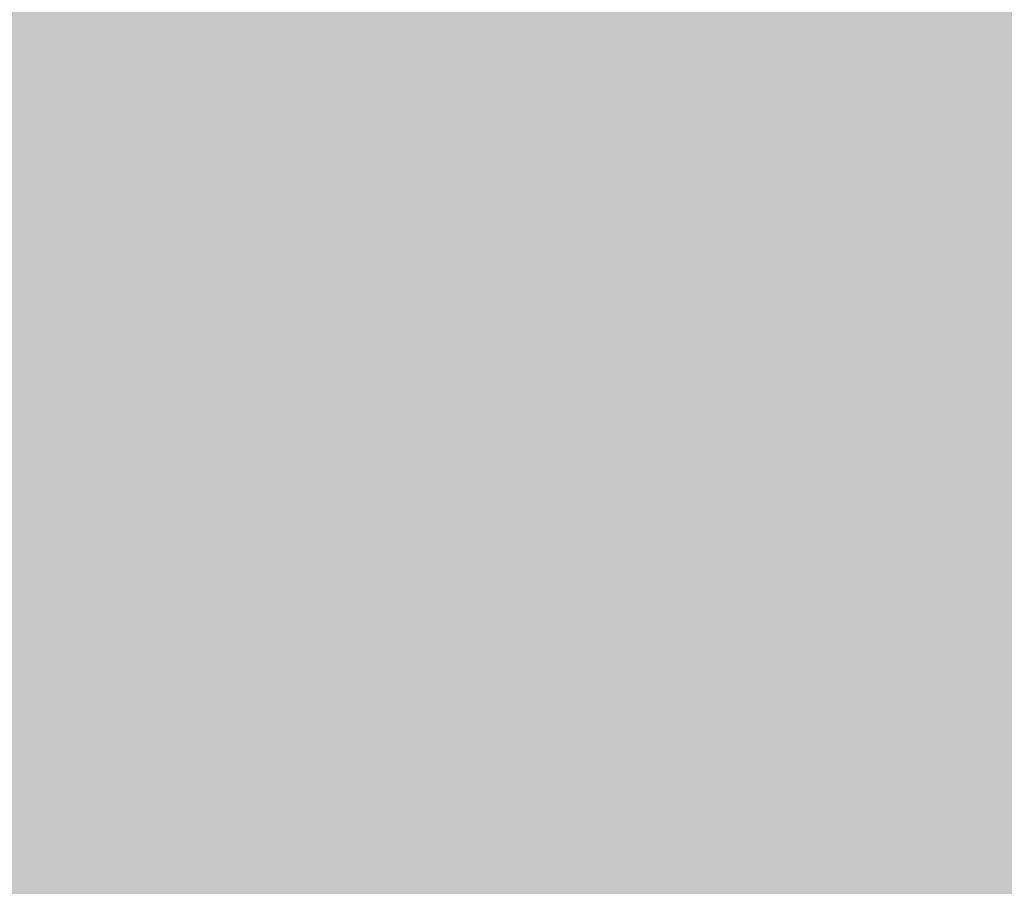
# Model space of a CAD drawing. Units: feet. Extents: x 3168 to 4724, y 827 to 1477.
# Tile 99 of 256: x 3277.376 to 3284.479, y 1087.401 to 1093.654. Entities that reach past the tile are written whole.
import ezdxf

# ---------------------------------------------------------------- set-up
doc = ezdxf.new("R2010")
doc.units = ezdxf.units.FT
doc.layers.add('A-ELEV-PATT', color=8, linetype='Continuous', lineweight=13)

msp = doc.modelspace()

# ---------------------------------------------------------------- hatches: boundary and pattern name
at = {"layer": 'A-ELEV-PATT'}
h = msp.add_hatch(color=256, dxfattribs=at)
h.dxf.hatch_style = 1
edge = h.paths.add_edge_path()
edge.add_ellipse((3552.9058, 979.2201), major_axis=(36.7449, 0), ratio=0.4848485, start_angle=0, end_angle=360)
edge = h.paths.add_edge_path()
edge.add_ellipse((3559.8916, 929.2523), major_axis=(36.7449, 0), ratio=0.4848485, start_angle=0, end_angle=360)
edge = h.paths.add_edge_path()
edge.add_line((3299.3168, 1198.6061), (3479.9167, 1198.6061))
edge.add_line((3479.9167, 1198.6061), (3479.9167, 1209.8686))
edge.add_spline(control_points=[(3479.9167, 1209.8686), (3464.3012, 1209.8686), (3448.6856, 1209.8686), (3410.9491, 1209.8686), (3388.8282, 1209.8686), (3355.6469, 1209.8686), (3344.5864, 1209.8686), (3327.9957, 1209.8686), (3322.4655, 1209.8686), (3314.1702, 1209.8686), (3311.4051, 1209.8686), (3307.2574, 1209.8686), (3305.8748, 1209.8686), (3303.801, 1209.8686), (3303.1097, 1209.8686), (3302.0728, 1209.8686), (3301.7272, 1209.8686), (3301.2087, 1209.8686), (3301.0359, 1209.8686), (3300.7767, 1209.8686), (3300.6903, 1209.8686), (3300.5606, 1209.8686), (3300.5174, 1209.8686), (3300.4526, 1209.8686), (3300.431, 1209.8686), (3300.3986, 1209.8686), (3300.3878, 1209.8686), (3300.3662, 1209.8686), (3300.3457, 1209.8686), (3300.3455, 1209.8686), (3300.3455, 1209.8686), (3300.3433, 1209.8686), (3300.3411, 1209.8686), (3300.3379, 1209.8686), (3300.3368, 1209.8686), (3300.3339, 1209.8686), (3300.3321, 1209.8686), (3300.3255, 1209.8686), (3300.3207, 1209.8686), (3300.3109, 1209.8686), (3300.306, 1209.8686), (3300.2905, 1209.8686), (3300.28, 1209.8686), (3300.2324, 1209.8688), (3300.1953, 1209.869), (3299.9511, 1209.8706), (3299.7448, 1209.8743), (3299.4368, 1209.8833), (3299.3344, 1209.8868), (3299.1811, 1209.8929), (3299.13, 1209.8951), (3298.6522, 1209.9168), (3298.2295, 1209.9457), (3297.6016, 1210.0024), (3297.3934, 1210.0235), (3297.0827, 1210.0583), (3296.9793, 1210.0705), (3296.293, 1210.1549), (3295.7181, 1210.2434), (3294.8687, 1210.3989), (3294.5877, 1210.4545), (3294.1693, 1210.5433), (3294.0304, 1210.5739), (3291.7071, 1211.1012), (3289.6536, 1211.8134), (3285.7763, 1213.564), (3283.9514, 1214.6035), (3280.5122, 1216.9801), (3278.8972, 1218.3176), (3276.3799, 1220.8295), (3275.416, 1221.9177), (3274.0393, 1223.7077), (3273.581, 1224.3495), (3273.1432, 1225.0163)], knot_values=[39.119033, 39.119033, 39.119033, 39.119033, 39.286353, 39.286353, 39.523379, 39.523379, 39.641892, 39.641892, 39.701148, 39.701148, 39.730777, 39.730777, 39.745591, 39.745591, 39.752998, 39.752998, 39.756701, 39.756701, 39.758553, 39.758553, 39.759479, 39.759479, 39.759942, 39.759942, 39.760173, 39.760173, 39.760289, 39.760289, 39.760405, 39.760405, 39.760463, 39.760463, 39.763389, 39.763389, 39.764851, 39.764851, 39.767304, 39.767304, 39.773825, 39.773825, 39.78057, 39.78057, 39.79477, 39.79477, 39.845194, 39.845194, 40.126715, 40.126715, 40.267476, 40.267476, 40.337856, 40.337856, 40.927023, 40.927023, 41.221606, 41.221606, 41.368898, 41.368898, 42.202622, 42.202622, 42.619485, 42.619485, 42.827916, 42.827916, 46.118323, 46.118323, 49.408731, 49.408731, 52.699139, 52.699139, 54.927489, 54.927489, 56.104228, 56.104228, 56.104228, 56.104228], weights=[1, 1, 1, 1, 1, 1, 1, 1, 1, 1, 1, 1, 1, 1, 1, 1, 1, 1, 1, 1, 1, 1, 1, 1, 1, 1, 1, 1, 1, 1, 1, 1, 1, 1, 1, 1, 1, 1, 1, 1, 1, 1, 1, 1, 1, 1, 1, 1, 1, 1, 1, 1, 1, 1, 1, 1, 1, 1, 1, 1, 1, 1, 1, 1, 1, 1, 1, 1, 1, 1, 1, 1, 1, 1], degree=3, periodic=0)
edge.add_line((3273.1432, 1225.0163), (3273.1432, 1099.0163))
edge.add_line((3273.1432, 1099.0163), (3299.3168, 1099.0163))
edge.add_line((3299.3168, 1099.0163), (3299.3168, 1198.6061))
edge = h.paths.add_edge_path()
edge.add_line((3304.7584, 1324.1581), (3479.9167, 1324.1581))
edge.add_line((3479.9167, 1324.1581), (3479.9167, 1335.7146))
edge.add_line((3479.9167, 1335.7146), (3269.1616, 1335.7146))
edge.add_spline(control_points=[(3269.1616, 1335.7146), (3264.0242, 1335.7146), (3258.3641, 1328.9582), (3259.2643, 1323.9003)], knot_values=[0, 0, 0, 0, 15.412191, 15.412191, 15.412191, 15.412191], degree=3, periodic=0)
edge.add_line((3259.2643, 1323.9003), (3265.5168, 1288.7691))
edge.add_line((3265.5168, 1288.7691), (3275.2651, 1261.5456))
edge.add_line((3275.2651, 1261.5456), (3304.7584, 1261.5456))
edge.add_line((3304.7584, 1261.5456), (3304.7584, 1324.1581))
h = msp.add_hatch(color=256, dxfattribs=at)
h.dxf.hatch_style = 1
h.paths.add_polyline_path([(3384.5252, 1099.0163), (3335.0292, 1099.0163), (3299.3168, 1099.0163), (3273.1432, 1099.0163), (3217.5654, 1099.0163), (3168.0693, 827.1163), (3335.0292, 827.1163)])

doc.saveas('drawing.dxf')
